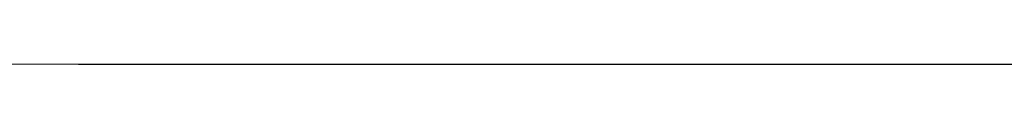
# Model space of a CAD drawing. Units: inches. Extents: x 459864 to 460310, y 324185 to 324787.
# Tile 97 of 112: x 460247.676 to 460248.739, y 324283.483 to 324283.483. Entities that reach past the tile are written whole.
import ezdxf

# ---------------------------------------------------------------- set-up
doc = ezdxf.new("R2010")
doc.units = ezdxf.units.IN
for name, color, linetype, lineweight in [('A-ANNO-DIMS', 2, 'Continuous', 18), ('L-HRDS', 9, 'Continuous', 18), ('L-SITE-PATT', 252, 'Continuous', 13)]:
    doc.layers.add(name, color=color, linetype=linetype, lineweight=lineweight)
doc.styles.get("Standard").update_dxf_attribs({"font": 'arial.ttf'})
doc.dimstyles.new('ISO-25', dxfattribs={"dimtxt": 6, "dimasz": 2.5, "dimexe": 1.25, "dimexo": 0.625, "dimtad": 1, "dimdec": 1, "dimlunit": 3, "dimtxsty": 'Standard', "dimcen": 2.5, "dimadec": 0, "dimazin": 0, "dimtfac": 1, "dimtdec": 1, "dimtmove": 0, "dimatfit": 3, "dimfxl": 1, "dimarcsym": 0})

# ---------------------------------------------------------------- blocks, each defined once
blk = doc.blocks.new('*D21')
at = {"layer": 'A-ANNO-DIMS', "color": 0, "lineweight": -2, "transparency": 16777216}
for p, q in [((460247.7399, 324715.4832), (460309.5804, 324715.4832)), ((460308.3304, 324712.9832), (460308.3304, 324285.9832)), ((460247.7399, 324283.4832), (460309.5804, 324283.4832))]:
    blk.add_line(p, q, dxfattribs=at)
at = {"layer": 'A-ANNO-DIMS', "color": 0, "transparency": 16777216}
for points in [[(460307.9137, 324712.9832), (460308.747, 324712.9832), (460308.3304, 324715.4832)], [(460307.9137, 324285.9832), (460308.747, 324285.9832), (460308.3304, 324283.4832)]]:
    blk.add_solid(points, dxfattribs=at)
at = {"layer": 'Defpoints', "color": 0, "transparency": 16777216}
for p in [(460247.1149, 324715.4832), (460247.1149, 324283.4832), (460308.3304, 324283.4832)]:
    blk.add_point(p, dxfattribs=at)
at = {"layer": 'A-ANNO-DIMS', "color": 0, "transparency": 16777216, "insert": (460304.6399, 324499.4832), "char_height": 6, "attachment_point": 5, "rotation": 90}
blk.add_mtext("36'", dxfattribs=at)

msp = doc.modelspace()

# ---------------------------------------------------------------- hatches: boundary and pattern name
at = {"layer": 'L-SITE-PATT'}
h = msp.add_hatch(dxfattribs=at)
h.set_pattern_fill('DOTS', color=256)
h.paths.add_polyline_path([(460269.8036, 324283.4832), (460247.1149, 324283.4832), (460121.9293, 324283.4832), (460121.9293, 324252.473), (460117.4293, 324252.473), (460110.1236, 324252.473), (460110.1236, 324243.2865), (460080.8295, 324243.2865), (460080.8295, 324252.473), (460061.1149, 324252.473), (460061.1149, 324251.8824), (460077.9089, 324251.8824), (460077.9089, 324199.4832), (460080.8295, 324199.4832), (460080.8295, 324207.5532), (460110.1236, 324207.5532), (460110.1236, 324199.4832), (460110.8133, 324199.4832), (460262.1149, 324199.4832), (460269.8036, 324199.4832)], flags=17)
edge = h.paths.add_edge_path(flags=0)
edge.add_ellipse((460222.5903, 324263.8132), major_axis=(-8.4853, 8.4853), ratio=1, start_angle=405, end_angle=495, ccw=False)
edge.add_line((460214.8209, 324254.6599), (460214.8316, 324254.6659))
edge.add_ellipse((460222.5903, 324263.8132), major_axis=(-8.4853, 8.4853), ratio=1, start_angle=405, end_angle=495, ccw=False)
edge.add_line((460210.7589, 324261.7806), (460210.7676, 324261.7868))
edge.add_ellipse((460222.5903, 324263.8132), major_axis=(-8.4853, 8.4853), ratio=1, start_angle=405, end_angle=495, ccw=False)
edge.add_ellipse((460222.5903, 324263.8132), major_axis=(-8.4853, 8.4853), ratio=1, start_angle=392.75402, end_angle=405, ccw=False)
edge.add_ellipse((460222.5903, 324263.8132), major_axis=(-8.4853, 8.4853), ratio=1, start_angle=380.93472, end_angle=392.75402, ccw=False)
edge.add_line((460211.3371, 324267.985), (460211.3404, 324267.985))
edge.add_ellipse((460222.5903, 324263.8132), major_axis=(-8.4853, 8.4853), ratio=1, start_angle=380.93472, end_angle=392.75402, ccw=False)
edge.add_ellipse((460222.5903, 324263.8132), major_axis=(-8.4853, 8.4853), ratio=1, start_angle=347.90152, end_angle=380.93472, ccw=False)
edge.add_ellipse((460222.5903, 324263.8132), major_axis=(-8.4853, 8.4853), ratio=1, start_angle=327.06192, end_angle=347.90152, ccw=False)
edge.add_ellipse((460222.5903, 324263.8132), major_axis=(-8.4853, 8.4853), ratio=1, start_angle=278.32464, end_angle=327.06192, ccw=False)
edge.add_line((460225.1583, 324275.536), (460225.1577, 324275.5346))
edge.add_ellipse((460222.5903, 324263.8132), major_axis=(-8.4853, 8.4853), ratio=1, start_angle=278.32464, end_angle=327.06192, ccw=False)
edge.add_ellipse((460222.5903, 324263.8132), major_axis=(-8.4853, 8.4853), ratio=1, start_angle=260.64357, end_angle=278.32464, ccw=False)
edge.add_ellipse((460222.5903, 324263.8132), major_axis=(-8.4853, 8.4853), ratio=1, start_angle=225, end_angle=260.64357, ccw=False)
edge.add_line((460234.5088, 324265.2428), (460234.5015, 324265.2394))
edge.add_ellipse((460222.5903, 324263.8132), major_axis=(-8.4853, 8.4853), ratio=1, start_angle=225, end_angle=260.64357, ccw=False)
edge.add_ellipse((460222.5903, 324263.8132), major_axis=(-8.4853, 8.4853), ratio=1, start_angle=495, end_angle=585, ccw=False)
edge.add_line((460234.4367, 324261.8612), (460234.4238, 324261.8578))
edge.add_ellipse((460222.5903, 324263.8132), major_axis=(-8.4853, 8.4853), ratio=1, start_angle=495, end_angle=585, ccw=False)
edge.add_line((460227.9501, 324253.0672), (460227.9464, 324253.0831))
edge.add_ellipse((460222.5903, 324263.8132), major_axis=(-8.4853, 8.4853), ratio=1, start_angle=495, end_angle=585, ccw=False)
edge.add_line((460226.223, 324252.3693), (460226.211, 324252.3796))
edge.add_ellipse((460222.5903, 324263.8132), major_axis=(-8.4853, 8.4853), ratio=1, start_angle=495, end_angle=585, ccw=False)
h.paths.add_polyline_path([(460219.6515, 324254.3467), (460218.4613, 324253.545), (460218.2754, 324254.7893), (460219.6424, 324256.5418), (460219.6246, 324260.8476), (460216.1101, 324257.333), (460214.35, 324256.9781), (460215.4164, 324259.3557), (460212.5239, 324258.4958), (460213.1373, 324259.9298), (460218.5072, 324263.8132), (460222.5903, 324263.8132), (460222.5903, 324267.8067), (460218.1755, 324272.2123), (460219.026, 324274.639), (460222.5903, 324272.8111), (460222.5903, 324275.4233), (460223.0571, 324274.8249), (460222.6752, 324273.4922), (460225.9117, 324267.1346), (460219.6246, 324260.8476)], flags=0)
edge = h.paths.add_edge_path(flags=0)
edge.add_ellipse((460194.5758, 324264.0465), major_axis=(-8.4853, 8.4853), ratio=1, start_angle=495, end_angle=585, ccw=False)
edge.add_line((460199.9356, 324253.3005), (460199.9319, 324253.3164))
edge.add_ellipse((460194.5758, 324264.0465), major_axis=(-8.4853, 8.4853), ratio=1, start_angle=495, end_angle=585, ccw=False)
edge.add_line((460198.2084, 324252.6025), (460198.1965, 324252.6128))
edge.add_ellipse((460194.5758, 324264.0465), major_axis=(-8.4853, 8.4853), ratio=1, start_angle=495, end_angle=585, ccw=False)
edge.add_ellipse((460194.5758, 324264.0465), major_axis=(-8.4853, 8.4853), ratio=1, start_angle=405, end_angle=495, ccw=False)
edge.add_line((460186.8063, 324254.8932), (460186.8171, 324254.8992))
edge.add_ellipse((460194.5758, 324264.0465), major_axis=(-8.4853, 8.4853), ratio=1, start_angle=405, end_angle=495, ccw=False)
edge.add_line((460182.7444, 324262.0138), (460182.753, 324262.0201))
edge.add_ellipse((460194.5758, 324264.0465), major_axis=(-8.4853, 8.4853), ratio=1, start_angle=405, end_angle=495, ccw=False)
edge.add_ellipse((460194.5758, 324264.0465), major_axis=(-8.4853, 8.4853), ratio=1, start_angle=392.75402, end_angle=405, ccw=False)
edge.add_ellipse((460194.5758, 324264.0465), major_axis=(-8.4853, 8.4853), ratio=1, start_angle=380.93472, end_angle=392.75402, ccw=False)
edge.add_line((460183.3225, 324268.2183), (460183.3259, 324268.2183))
edge.add_ellipse((460194.5758, 324264.0465), major_axis=(-8.4853, 8.4853), ratio=1, start_angle=380.93472, end_angle=392.75402, ccw=False)
edge.add_ellipse((460194.5758, 324264.0465), major_axis=(-8.4853, 8.4853), ratio=1, start_angle=347.90152, end_angle=380.93472, ccw=False)
edge.add_ellipse((460194.5758, 324264.0465), major_axis=(-8.4853, 8.4853), ratio=1, start_angle=327.06192, end_angle=347.90152, ccw=False)
edge.add_ellipse((460194.5758, 324264.0465), major_axis=(-8.4853, 8.4853), ratio=1, start_angle=278.32464, end_angle=327.06192, ccw=False)
edge.add_line((460197.1437, 324275.7693), (460197.1432, 324275.7679))
edge.add_ellipse((460194.5758, 324264.0465), major_axis=(-8.4853, 8.4853), ratio=1, start_angle=278.32464, end_angle=327.06192, ccw=False)
edge.add_ellipse((460194.5758, 324264.0465), major_axis=(-8.4853, 8.4853), ratio=1, start_angle=260.64357, end_angle=278.32464, ccw=False)
edge.add_ellipse((460194.5758, 324264.0465), major_axis=(-8.4853, 8.4853), ratio=1, start_angle=225, end_angle=260.64357, ccw=False)
edge.add_line((460206.4943, 324265.4761), (460206.4869, 324265.4727))
edge.add_ellipse((460194.5758, 324264.0465), major_axis=(-8.4853, 8.4853), ratio=1, start_angle=225, end_angle=260.64357, ccw=False)
edge.add_ellipse((460194.5758, 324264.0465), major_axis=(-8.4853, 8.4853), ratio=1, start_angle=495, end_angle=585, ccw=False)
edge.add_line((460206.4221, 324262.0945), (460206.4092, 324262.0911))
h.paths.add_polyline_path([(460191.6101, 324261.0808), (460191.6369, 324254.5799), (460190.4468, 324253.7783), (460190.2609, 324255.0226), (460191.6279, 324256.775), (460191.6101, 324261.0808), (460188.0956, 324257.5663), (460186.3354, 324257.2113), (460187.4018, 324259.5889), (460184.5094, 324258.7291), (460185.1228, 324260.1631), (460190.4927, 324264.0465), (460194.5758, 324264.0465), (460194.5758, 324268.04), (460190.161, 324272.4456), (460191.0114, 324274.8722), (460194.5758, 324273.0444), (460194.5758, 324275.6566), (460195.0426, 324275.0582), (460194.6607, 324273.7255), (460197.8971, 324267.3679)], flags=0)
edge = h.paths.add_edge_path(flags=0)
edge.add_ellipse((460252.912, 324263.5776), major_axis=(-8.4853, 8.4853), ratio=1, start_angle=405, end_angle=495, ccw=False)
edge.add_line((460241.0806, 324261.5449), (460241.0892, 324261.5512))
edge.add_ellipse((460252.912, 324263.5776), major_axis=(-8.4853, 8.4853), ratio=1, start_angle=405, end_angle=495, ccw=False)
edge.add_ellipse((460252.912, 324263.5776), major_axis=(-8.4853, 8.4853), ratio=1, start_angle=392.75402, end_angle=405, ccw=False)
edge.add_ellipse((460252.912, 324263.5776), major_axis=(-8.4853, 8.4853), ratio=1, start_angle=380.93472, end_angle=392.75402, ccw=False)
edge.add_line((460241.6587, 324267.7494), (460241.6621, 324267.7494))
edge.add_ellipse((460252.912, 324263.5776), major_axis=(-8.4853, 8.4853), ratio=1, start_angle=380.93472, end_angle=392.75402, ccw=False)
edge.add_ellipse((460252.912, 324263.5776), major_axis=(-8.4853, 8.4853), ratio=1, start_angle=347.90152, end_angle=380.93472, ccw=False)
edge.add_ellipse((460252.912, 324263.5776), major_axis=(-8.4853, 8.4853), ratio=1, start_angle=327.06192, end_angle=347.90152, ccw=False)
edge.add_ellipse((460252.912, 324263.5776), major_axis=(-8.4853, 8.4853), ratio=1, start_angle=278.32464, end_angle=327.06192, ccw=False)
edge.add_line((460255.4799, 324275.3004), (460255.4794, 324275.299))
edge.add_ellipse((460252.912, 324263.5776), major_axis=(-8.4853, 8.4853), ratio=1, start_angle=278.32464, end_angle=327.06192, ccw=False)
edge.add_ellipse((460252.912, 324263.5776), major_axis=(-8.4853, 8.4853), ratio=1, start_angle=260.64357, end_angle=278.32464, ccw=False)
edge.add_ellipse((460252.912, 324263.5776), major_axis=(-8.4853, 8.4853), ratio=1, start_angle=225, end_angle=260.64357, ccw=False)
edge.add_line((460264.8305, 324265.0072), (460264.8231, 324265.0038))
edge.add_ellipse((460252.912, 324263.5776), major_axis=(-8.4853, 8.4853), ratio=1, start_angle=225, end_angle=260.64357, ccw=False)
edge.add_ellipse((460252.912, 324263.5776), major_axis=(-8.4853, 8.4853), ratio=1, start_angle=495, end_angle=585, ccw=False)
edge.add_line((460264.7583, 324261.6256), (460264.7454, 324261.6222))
edge.add_ellipse((460252.912, 324263.5776), major_axis=(-8.4853, 8.4853), ratio=1, start_angle=495, end_angle=585, ccw=False)
edge.add_line((460258.2718, 324252.8316), (460258.2681, 324252.8475))
edge.add_ellipse((460252.912, 324263.5776), major_axis=(-8.4853, 8.4853), ratio=1, start_angle=495, end_angle=585, ccw=False)
edge.add_line((460256.5446, 324252.1337), (460256.5327, 324252.1439))
edge.add_ellipse((460252.912, 324263.5776), major_axis=(-8.4853, 8.4853), ratio=1, start_angle=495, end_angle=585, ccw=False)
edge.add_ellipse((460252.912, 324263.5776), major_axis=(-8.4853, 8.4853), ratio=1, start_angle=405, end_angle=495, ccw=False)
edge.add_line((460245.1425, 324254.4243), (460245.1533, 324254.4303))
h.paths.add_polyline_path([(460244.6716, 324256.7425), (460245.738, 324259.1201), (460242.8456, 324258.2602), (460243.459, 324259.6942), (460248.8289, 324263.5776), (460252.912, 324263.5776), (460252.912, 324267.5711), (460248.4972, 324271.9767), (460249.3476, 324274.4034), (460252.912, 324272.5755), (460252.912, 324275.1877), (460253.3788, 324274.5893), (460252.9969, 324273.2566), (460256.2333, 324266.899), (460249.9463, 324260.612), (460249.9731, 324254.111), (460248.783, 324253.3094), (460248.5971, 324254.5537), (460249.9641, 324256.3062), (460249.9463, 324260.612), (460246.4318, 324257.0974)], flags=0)
edge = h.paths.add_edge_path(flags=0)
edge.add_ellipse((460167.4387, 324262.8328), major_axis=(-8.4853, 8.4853), ratio=1, start_angle=495, end_angle=585, ccw=False)
edge.add_line((460172.7985, 324252.0868), (460172.7948, 324252.1027))
edge.add_ellipse((460167.4387, 324262.8328), major_axis=(-8.4853, 8.4853), ratio=1, start_angle=495, end_angle=585, ccw=False)
edge.add_line((460171.0714, 324251.3888), (460171.0594, 324251.3991))
edge.add_ellipse((460167.4387, 324262.8328), major_axis=(-8.4853, 8.4853), ratio=1, start_angle=495, end_angle=585, ccw=False)
edge.add_ellipse((460167.4387, 324262.8328), major_axis=(-8.4853, 8.4853), ratio=1, start_angle=405, end_angle=495, ccw=False)
edge.add_line((460159.6693, 324253.6795), (460159.68, 324253.6855))
edge.add_ellipse((460167.4387, 324262.8328), major_axis=(-8.4853, 8.4853), ratio=1, start_angle=405, end_angle=495, ccw=False)
edge.add_line((460155.6073, 324260.8001), (460155.616, 324260.8064))
edge.add_ellipse((460167.4387, 324262.8328), major_axis=(-8.4853, 8.4853), ratio=1, start_angle=405, end_angle=495, ccw=False)
edge.add_ellipse((460167.4387, 324262.8328), major_axis=(-8.4853, 8.4853), ratio=1, start_angle=392.75402, end_angle=405, ccw=False)
edge.add_ellipse((460167.4387, 324262.8328), major_axis=(-8.4853, 8.4853), ratio=1, start_angle=380.93472, end_angle=392.75402, ccw=False)
edge.add_line((460156.1855, 324267.0046), (460156.1888, 324267.0046))
edge.add_ellipse((460167.4387, 324262.8328), major_axis=(-8.4853, 8.4853), ratio=1, start_angle=380.93472, end_angle=392.75402, ccw=False)
edge.add_ellipse((460167.4387, 324262.8328), major_axis=(-8.4853, 8.4853), ratio=1, start_angle=347.90152, end_angle=380.93472, ccw=False)
edge.add_ellipse((460167.4387, 324262.8328), major_axis=(-8.4853, 8.4853), ratio=1, start_angle=327.06192, end_angle=347.90152, ccw=False)
edge.add_ellipse((460167.4387, 324262.8328), major_axis=(-8.4853, 8.4853), ratio=1, start_angle=278.32464, end_angle=327.06192, ccw=False)
edge.add_line((460170.0067, 324274.5556), (460170.0061, 324274.5542))
edge.add_ellipse((460167.4387, 324262.8328), major_axis=(-8.4853, 8.4853), ratio=1, start_angle=278.32464, end_angle=327.06192, ccw=False)
edge.add_ellipse((460167.4387, 324262.8328), major_axis=(-8.4853, 8.4853), ratio=1, start_angle=260.64357, end_angle=278.32464, ccw=False)
edge.add_ellipse((460167.4387, 324262.8328), major_axis=(-8.4853, 8.4853), ratio=1, start_angle=225, end_angle=260.64357, ccw=False)
edge.add_line((460179.3572, 324264.2624), (460179.3499, 324264.259))
edge.add_ellipse((460167.4387, 324262.8328), major_axis=(-8.4853, 8.4853), ratio=1, start_angle=225, end_angle=260.64357, ccw=False)
edge.add_ellipse((460167.4387, 324262.8328), major_axis=(-8.4853, 8.4853), ratio=1, start_angle=495, end_angle=585, ccw=False)
edge.add_line((460179.2851, 324260.8808), (460179.2722, 324260.8774))
h.paths.add_polyline_path([(460164.473, 324259.8671), (460164.4998, 324253.3662), (460163.3097, 324252.5645), (460163.1238, 324253.8089), (460164.4908, 324255.5613), (460164.473, 324259.8671), (460160.9585, 324256.3526), (460159.1984, 324255.9976), (460160.2648, 324258.3752), (460157.3723, 324257.5154), (460157.9857, 324258.9494), (460163.3556, 324262.8328), (460167.4387, 324262.8328), (460167.4387, 324266.8263), (460163.0239, 324271.2319), (460163.8744, 324273.6585), (460167.4387, 324271.8307), (460167.4387, 324274.4429), (460167.9055, 324273.8445), (460167.5236, 324272.5118), (460170.7601, 324266.1542)], flags=0)
edge = h.paths.add_edge_path(flags=0)
edge.add_ellipse((460140.7581, 324262.3696), major_axis=(-8.4853, 8.4853), ratio=1, start_angle=495, end_angle=585, ccw=False)
edge.add_line((460146.1179, 324251.6235), (460146.1142, 324251.6395))
edge.add_ellipse((460140.7581, 324262.3696), major_axis=(-8.4853, 8.4853), ratio=1, start_angle=495, end_angle=585, ccw=False)
edge.add_line((460144.3908, 324250.9256), (460144.3788, 324250.9359))
edge.add_ellipse((460140.7581, 324262.3696), major_axis=(-8.4853, 8.4853), ratio=1, start_angle=495, end_angle=585, ccw=False)
edge.add_ellipse((460140.7581, 324262.3696), major_axis=(-8.4853, 8.4853), ratio=1, start_angle=405, end_angle=495, ccw=False)
edge.add_line((460132.9887, 324253.2162), (460132.9994, 324253.2223))
edge.add_ellipse((460140.7581, 324262.3696), major_axis=(-8.4853, 8.4853), ratio=1, start_angle=405, end_angle=495, ccw=False)
edge.add_line((460128.9267, 324260.3369), (460128.9354, 324260.3432))
edge.add_ellipse((460140.7581, 324262.3696), major_axis=(-8.4853, 8.4853), ratio=1, start_angle=405, end_angle=495, ccw=False)
edge.add_ellipse((460140.7581, 324262.3696), major_axis=(-8.4853, 8.4853), ratio=1, start_angle=392.75402, end_angle=405, ccw=False)
edge.add_ellipse((460140.7581, 324262.3696), major_axis=(-8.4853, 8.4853), ratio=1, start_angle=380.93472, end_angle=392.75402, ccw=False)
edge.add_line((460129.5049, 324266.5414), (460129.5082, 324266.5414))
edge.add_ellipse((460140.7581, 324262.3696), major_axis=(-8.4853, 8.4853), ratio=1, start_angle=380.93472, end_angle=392.75402, ccw=False)
edge.add_ellipse((460140.7581, 324262.3696), major_axis=(-8.4853, 8.4853), ratio=1, start_angle=347.90152, end_angle=380.93472, ccw=False)
edge.add_ellipse((460140.7581, 324262.3696), major_axis=(-8.4853, 8.4853), ratio=1, start_angle=327.06192, end_angle=347.90152, ccw=False)
edge.add_ellipse((460140.7581, 324262.3696), major_axis=(-8.4853, 8.4853), ratio=1, start_angle=278.32464, end_angle=327.06192, ccw=False)
edge.add_line((460143.3261, 324274.0923), (460143.3255, 324274.091))
edge.add_ellipse((460140.7581, 324262.3696), major_axis=(-8.4853, 8.4853), ratio=1, start_angle=278.32464, end_angle=327.06192, ccw=False)
edge.add_ellipse((460140.7581, 324262.3696), major_axis=(-8.4853, 8.4853), ratio=1, start_angle=260.64357, end_angle=278.32464, ccw=False)
edge.add_ellipse((460140.7581, 324262.3696), major_axis=(-8.4853, 8.4853), ratio=1, start_angle=225, end_angle=260.64357, ccw=False)
edge.add_line((460152.6766, 324263.7992), (460152.6692, 324263.7958))
edge.add_ellipse((460140.7581, 324262.3696), major_axis=(-8.4853, 8.4853), ratio=1, start_angle=225, end_angle=260.64357, ccw=False)
edge.add_ellipse((460140.7581, 324262.3696), major_axis=(-8.4853, 8.4853), ratio=1, start_angle=495, end_angle=585, ccw=False)
edge.add_line((460152.6045, 324260.4176), (460152.5916, 324260.4142))
h.paths.add_polyline_path([(460137.7924, 324259.4039), (460137.8192, 324252.903), (460136.6291, 324252.1013), (460136.4432, 324253.3457), (460137.8102, 324255.0981), (460137.7924, 324259.4039), (460134.2779, 324255.8894), (460132.5178, 324255.5344), (460133.5842, 324257.912), (460130.6917, 324257.0522), (460131.3051, 324258.4862), (460136.675, 324262.3696), (460140.7581, 324262.3696), (460140.7581, 324266.3631), (460136.3433, 324270.7687), (460137.1938, 324273.1953), (460140.7581, 324271.3675), (460140.7581, 324273.9797), (460141.2249, 324273.3813), (460140.843, 324272.0486), (460144.0795, 324265.691)], flags=0)
h.paths.add_polyline_path([(460110.1236, 324227.4139), (460080.8295, 324227.4139), (460080.8295, 324235.4839), (460110.1236, 324235.4839)], flags=16)
h.paths.add_polyline_path([(460110.1236, 324220.7966), (460110.1236, 324212.7267), (460080.8295, 324212.7267), (460080.8295, 324220.7966)], flags=16)
h.paths.add_polyline_path([(460269.8036, 324283.4832), (460247.1149, 324283.4832), (460121.9293, 324283.4832), (460121.9293, 324252.473), (460117.4293, 324252.473), (460110.1236, 324252.473), (460110.1236, 324243.2865), (460080.8295, 324243.2865), (460080.8295, 324252.473), (460061.1149, 324252.473), (460061.1149, 324251.8824), (460077.9089, 324251.8824), (460077.9089, 324199.4832), (460080.8295, 324199.4832), (460080.8295, 324207.5532), (460110.1236, 324207.5532), (460110.1236, 324199.4832), (460262.1149, 324199.4832), (460269.8036, 324199.4832)], flags=17)
h.paths.add_polyline_path([(460219.6515, 324254.3467), (460218.4613, 324253.545), (460218.2754, 324254.7893), (460219.6424, 324256.5418), (460219.6246, 324260.8476), (460216.1101, 324257.333), (460214.35, 324256.9781), (460215.4164, 324259.3557), (460212.5239, 324258.4958), (460213.1373, 324259.9298), (460218.5072, 324263.8132), (460222.5903, 324263.8132), (460220.1805, 324266.223), (460215.461, 324265.3076), (460211.8345, 324266.1366), (460216.2466, 324267.985), (460218.4185, 324267.985), (460222.5903, 324263.8132), (460222.5903, 324267.8067), (460218.1755, 324272.2123), (460219.026, 324274.639), (460222.5903, 324272.8111), (460222.5903, 324275.4233), (460223.0571, 324274.8249), (460222.6752, 324273.4922), (460225.9117, 324267.1346), (460222.5903, 324263.8132), (460231.3829, 324263.8132), (460228.4847, 324262.4878), (460224.4252, 324261.9783), (460228.6799, 324257.7236), (460228.9658, 324254.791), (460227.1418, 324256.5366), (460227.5421, 324254.8186), (460227.3333, 324253.6145), (460222.5903, 324259.9846), (460222.5903, 324255.4967), (460221.3774, 324256.5408), (460220.5758, 324261.7987), (460219.6246, 324260.8476)], flags=0)
h.paths.add_polyline_path([(460199.1272, 324256.7699), (460199.5275, 324255.0518), (460199.3188, 324253.8477), (460194.5758, 324260.2179), (460194.5758, 324255.7299), (460193.3629, 324256.7741), (460192.5613, 324262.032), (460191.6101, 324261.0808), (460191.6369, 324254.5799), (460190.4468, 324253.7783), (460190.2609, 324255.0226), (460191.6279, 324256.775), (460191.6101, 324261.0808), (460188.0956, 324257.5663), (460186.3354, 324257.2113), (460187.4018, 324259.5889), (460184.5094, 324258.7291), (460185.1228, 324260.1631), (460190.4927, 324264.0465), (460194.5758, 324264.0465), (460192.1659, 324266.4563), (460187.4464, 324265.5409), (460183.82, 324266.3698), (460188.2321, 324268.2183), (460190.404, 324268.2183), (460194.5758, 324264.0465), (460194.5758, 324268.04), (460190.161, 324272.4456), (460191.0114, 324274.8722), (460194.5758, 324273.0444), (460194.5758, 324275.6566), (460195.0426, 324275.0582), (460194.6607, 324273.7255), (460197.8971, 324267.3679), (460194.5758, 324264.0465), (460203.3683, 324264.0465), (460200.4702, 324262.7211), (460196.4107, 324262.2116), (460200.6654, 324257.9569), (460200.9513, 324255.0243)], flags=0)
h.paths.add_polyline_path([(460244.6716, 324256.7425), (460245.738, 324259.1201), (460242.8456, 324258.2602), (460243.459, 324259.6942), (460248.8289, 324263.5776), (460252.912, 324263.5776), (460250.5022, 324265.9874), (460245.7826, 324265.072), (460242.1562, 324265.9009), (460246.5683, 324267.7494), (460248.7402, 324267.7494), (460252.912, 324263.5776), (460252.912, 324267.5711), (460248.4972, 324271.9767), (460249.3476, 324274.4034), (460252.912, 324272.5755), (460252.912, 324275.1877), (460253.3788, 324274.5893), (460252.9969, 324273.2566), (460256.2333, 324266.899), (460252.912, 324263.5776), (460261.7045, 324263.5776), (460258.8064, 324262.2522), (460254.7469, 324261.7427), (460259.0016, 324257.488), (460259.2875, 324254.5554), (460257.4634, 324256.301), (460257.8637, 324254.583), (460257.655, 324253.3789), (460252.912, 324259.749), (460252.912, 324255.2611), (460251.6991, 324256.3052), (460250.8975, 324261.5631), (460249.9463, 324260.612), (460249.9731, 324254.111), (460248.783, 324253.3094), (460248.5971, 324254.5537), (460249.9641, 324256.3062), (460249.9463, 324260.612), (460246.4318, 324257.0974)], flags=0)
h.paths.add_polyline_path([(460173.5283, 324256.7432), (460173.8142, 324253.8106), (460171.9902, 324255.5562), (460172.3905, 324253.8381), (460172.1817, 324252.634), (460167.4387, 324259.0042), (460167.4387, 324254.5162), (460166.2258, 324255.5604), (460165.4242, 324260.8183), (460164.473, 324259.8671), (460164.4998, 324253.3662), (460163.3097, 324252.5645), (460163.1238, 324253.8089), (460164.4908, 324255.5613), (460164.473, 324259.8671), (460160.9585, 324256.3526), (460159.1984, 324255.9976), (460160.2648, 324258.3752), (460157.3723, 324257.5154), (460157.9857, 324258.9494), (460163.3556, 324262.8328), (460167.4387, 324262.8328), (460165.0289, 324265.2426), (460160.3094, 324264.3272), (460156.6829, 324265.1561), (460161.095, 324267.0046), (460163.2669, 324267.0046), (460167.4387, 324262.8328), (460167.4387, 324266.8263), (460163.0239, 324271.2319), (460163.8744, 324273.6585), (460167.4387, 324271.8307), (460167.4387, 324274.4429), (460167.9055, 324273.8445), (460167.5236, 324272.5118), (460170.7601, 324266.1542), (460167.4387, 324262.8328), (460176.2313, 324262.8328), (460173.3331, 324261.5074), (460169.2736, 324260.9979)], flags=0)
h.paths.add_polyline_path([(460146.8477, 324256.28), (460147.1336, 324253.3474), (460145.3096, 324255.093), (460145.7099, 324253.3749), (460145.5011, 324252.1708), (460140.7581, 324258.541), (460140.7581, 324254.053), (460139.5452, 324255.0972), (460138.7436, 324260.3551), (460137.7924, 324259.4039), (460137.8192, 324252.903), (460136.6291, 324252.1013), (460136.4432, 324253.3457), (460137.8102, 324255.0981), (460137.7924, 324259.4039), (460134.2779, 324255.8894), (460132.5178, 324255.5344), (460133.5842, 324257.912), (460130.6917, 324257.0522), (460131.3051, 324258.4862), (460136.675, 324262.3696), (460140.7581, 324262.3696), (460138.3483, 324264.7794), (460133.6288, 324263.864), (460130.0023, 324264.6929), (460134.4144, 324266.5414), (460136.5863, 324266.5414), (460140.7581, 324262.3696), (460140.7581, 324266.3631), (460136.3433, 324270.7687), (460137.1938, 324273.1953), (460140.7581, 324271.3675), (460140.7581, 324273.9797), (460141.2249, 324273.3813), (460140.843, 324272.0486), (460144.0795, 324265.691), (460140.7581, 324262.3696), (460149.5507, 324262.3696), (460146.6525, 324261.0442), (460142.593, 324260.5347)], flags=0)
edge = h.paths.add_edge_path()
edge.add_line((460269.8036, 324272.5491), (460260.8815, 324272.5491))
edge.add_ellipse((460252.912, 324263.5776), major_axis=(-8.4853, 8.4853), ratio=1, start_angle=260.64357, end_angle=273.38462, ccw=False)
edge.add_line((460262.2826, 324271.0921), (460262.2606, 324271.0911))
edge.add_ellipse((460252.912, 324263.5776), major_axis=(-8.4853, 8.4853), ratio=1, start_angle=260.64357, end_angle=273.38462, ccw=False)
edge.add_ellipse((460252.912, 324263.5776), major_axis=(-8.4853, 8.4853), ratio=1, start_angle=225, end_angle=260.64357, ccw=False)
edge.add_line((460263.6086, 324269.0633), (460263.5717, 324269.0583))
edge.add_ellipse((460252.912, 324263.5776), major_axis=(-8.4853, 8.4853), ratio=1, start_angle=225, end_angle=260.64357, ccw=False)
edge.add_line((460264.6155, 324266.3055), (460264.5854, 324266.3052))
edge.add_ellipse((460252.912, 324263.5776), major_axis=(-8.4853, 8.4853), ratio=1, start_angle=225, end_angle=260.64357, ccw=False)
edge.add_line((460264.8305, 324265.0072), (460264.8231, 324265.0038))
edge.add_ellipse((460252.912, 324263.5776), major_axis=(-8.4853, 8.4853), ratio=1, start_angle=225, end_angle=260.64357, ccw=False)
edge.add_ellipse((460252.912, 324263.5776), major_axis=(-8.4853, 8.4853), ratio=1, start_angle=495, end_angle=585, ccw=False)
edge.add_line((460264.7583, 324261.6256), (460264.7454, 324261.6222))
edge.add_ellipse((460252.912, 324263.5776), major_axis=(-8.4853, 8.4853), ratio=1, start_angle=495, end_angle=585, ccw=False)
edge.add_line((460263.4422, 324257.739), (460263.3893, 324257.7792))
edge.add_ellipse((460252.912, 324263.5776), major_axis=(-8.4853, 8.4853), ratio=1, start_angle=495, end_angle=585, ccw=False)
edge.add_line((460258.1281, 324252.7435), (460258.1019, 324252.7787))
edge.add_ellipse((460252.912, 324263.5776), major_axis=(-8.4853, 8.4853), ratio=1, start_angle=495, end_angle=585, ccw=False)
edge.add_line((460256.5446, 324252.1337), (460256.5327, 324252.1439))
edge.add_ellipse((460252.912, 324263.5776), major_axis=(-8.4853, 8.4853), ratio=1, start_angle=495, end_angle=585, ccw=False)
edge.add_ellipse((460252.912, 324263.5776), major_axis=(-8.4853, 8.4853), ratio=1, start_angle=405, end_angle=495, ccw=False)
edge.add_line((460250.594, 324251.7804), (460250.6047, 324251.8198))
edge.add_ellipse((460252.912, 324263.5776), major_axis=(-8.4853, 8.4853), ratio=1, start_angle=405, end_angle=495, ccw=False)
edge.add_line((460245.1425, 324254.4243), (460245.1533, 324254.4303))
edge.add_ellipse((460252.912, 324263.5776), major_axis=(-8.4853, 8.4853), ratio=1, start_angle=405, end_angle=495, ccw=False)
edge.add_line((460243.5246, 324256.059), (460243.5603, 324256.0914))
edge.add_ellipse((460252.912, 324263.5776), major_axis=(-8.4853, 8.4853), ratio=1, start_angle=405, end_angle=495, ccw=False)
edge.add_line((460241.4401, 324259.8927), (460241.5224, 324259.8959))
edge.add_ellipse((460252.912, 324263.5776), major_axis=(-8.4853, 8.4853), ratio=1, start_angle=405, end_angle=495, ccw=False)
edge.add_line((460241.0806, 324261.5449), (460241.0892, 324261.5512))
edge.add_ellipse((460252.912, 324263.5776), major_axis=(-8.4853, 8.4853), ratio=1, start_angle=405, end_angle=495, ccw=False)
edge.add_ellipse((460252.912, 324263.5776), major_axis=(-8.4853, 8.4853), ratio=1, start_angle=392.75402, end_angle=405, ccw=False)
edge.add_line((460241.0503, 324265.4376), (460241.0626, 324265.4428))
edge.add_ellipse((460252.912, 324263.5776), major_axis=(-8.4853, 8.4853), ratio=1, start_angle=392.75402, end_angle=405, ccw=False)
edge.add_ellipse((460252.912, 324263.5776), major_axis=(-8.4853, 8.4853), ratio=1, start_angle=380.93472, end_angle=392.75402, ccw=False)
edge.add_line((460241.4519, 324267.1764), (460241.469, 324267.171))
edge.add_ellipse((460252.912, 324263.5776), major_axis=(-8.4853, 8.4853), ratio=1, start_angle=380.93472, end_angle=392.75402, ccw=False)
edge.add_line((460241.6587, 324267.7494), (460241.6621, 324267.7494))
edge.add_ellipse((460252.912, 324263.5776), major_axis=(-8.4853, 8.4853), ratio=1, start_angle=380.93472, end_angle=392.75402, ccw=False)
edge.add_ellipse((460252.912, 324263.5776), major_axis=(-8.4853, 8.4853), ratio=1, start_angle=356.61538, end_angle=380.93472, ccw=False)
edge.add_line((460244.8803, 324272.4877), (460244.7127, 324272.5491))
edge.add_line((460244.7127, 324272.5491), (460230.8174, 324272.5491))
edge.add_ellipse((460222.5903, 324263.8132), major_axis=(-8.4853, 8.4853), ratio=1, start_angle=260.64357, end_angle=271.71777, ccw=False)
edge.add_ellipse((460222.5903, 324263.8132), major_axis=(-8.4853, 8.4853), ratio=1, start_angle=225, end_angle=260.64357, ccw=False)
edge.add_line((460233.2869, 324269.2989), (460233.25, 324269.2939))
edge.add_ellipse((460222.5903, 324263.8132), major_axis=(-8.4853, 8.4853), ratio=1, start_angle=225, end_angle=260.64357, ccw=False)
edge.add_line((460234.2938, 324266.5412), (460234.2637, 324266.5408))
edge.add_ellipse((460222.5903, 324263.8132), major_axis=(-8.4853, 8.4853), ratio=1, start_angle=225, end_angle=260.64357, ccw=False)
edge.add_line((460234.5088, 324265.2428), (460234.5015, 324265.2394))
edge.add_ellipse((460222.5903, 324263.8132), major_axis=(-8.4853, 8.4853), ratio=1, start_angle=225, end_angle=260.64357, ccw=False)
edge.add_ellipse((460222.5903, 324263.8132), major_axis=(-8.4853, 8.4853), ratio=1, start_angle=495, end_angle=585, ccw=False)
edge.add_line((460234.4367, 324261.8612), (460234.4238, 324261.8578))
edge.add_ellipse((460222.5903, 324263.8132), major_axis=(-8.4853, 8.4853), ratio=1, start_angle=495, end_angle=585, ccw=False)
edge.add_line((460233.1205, 324257.9746), (460233.0676, 324258.0149))
edge.add_ellipse((460222.5903, 324263.8132), major_axis=(-8.4853, 8.4853), ratio=1, start_angle=495, end_angle=585, ccw=False)
edge.add_line((460227.8064, 324252.9791), (460227.7802, 324253.0143))
edge.add_ellipse((460222.5903, 324263.8132), major_axis=(-8.4853, 8.4853), ratio=1, start_angle=495, end_angle=585, ccw=False)
edge.add_line((460226.223, 324252.3693), (460226.211, 324252.3796))
edge.add_ellipse((460222.5903, 324263.8132), major_axis=(-8.4853, 8.4853), ratio=1, start_angle=495, end_angle=585, ccw=False)
edge.add_ellipse((460222.5903, 324263.8132), major_axis=(-8.4853, 8.4853), ratio=1, start_angle=405, end_angle=495, ccw=False)
edge.add_line((460220.2723, 324252.016), (460220.283, 324252.0554))
edge.add_ellipse((460222.5903, 324263.8132), major_axis=(-8.4853, 8.4853), ratio=1, start_angle=405, end_angle=495, ccw=False)
edge.add_line((460214.8209, 324254.6599), (460214.8316, 324254.6659))
edge.add_ellipse((460222.5903, 324263.8132), major_axis=(-8.4853, 8.4853), ratio=1, start_angle=405, end_angle=495, ccw=False)
edge.add_line((460213.2029, 324256.2946), (460213.2387, 324256.327))
edge.add_ellipse((460222.5903, 324263.8132), major_axis=(-8.4853, 8.4853), ratio=1, start_angle=405, end_angle=495, ccw=False)
edge.add_line((460211.1184, 324260.1283), (460211.2008, 324260.1315))
edge.add_ellipse((460222.5903, 324263.8132), major_axis=(-8.4853, 8.4853), ratio=1, start_angle=405, end_angle=495, ccw=False)
edge.add_line((460210.7589, 324261.7806), (460210.7676, 324261.7868))
edge.add_ellipse((460222.5903, 324263.8132), major_axis=(-8.4853, 8.4853), ratio=1, start_angle=405, end_angle=495, ccw=False)
edge.add_ellipse((460222.5903, 324263.8132), major_axis=(-8.4853, 8.4853), ratio=1, start_angle=392.75402, end_angle=405, ccw=False)
edge.add_line((460210.7286, 324265.6732), (460210.7409, 324265.6784))
edge.add_ellipse((460222.5903, 324263.8132), major_axis=(-8.4853, 8.4853), ratio=1, start_angle=392.75402, end_angle=405, ccw=False)
edge.add_ellipse((460222.5903, 324263.8132), major_axis=(-8.4853, 8.4853), ratio=1, start_angle=380.93472, end_angle=392.75402, ccw=False)
edge.add_line((460211.1302, 324267.412), (460211.1474, 324267.4066))
edge.add_ellipse((460222.5903, 324263.8132), major_axis=(-8.4853, 8.4853), ratio=1, start_angle=380.93472, end_angle=392.75402, ccw=False)
edge.add_line((460211.3371, 324267.985), (460211.3404, 324267.985))
edge.add_ellipse((460222.5903, 324263.8132), major_axis=(-8.4853, 8.4853), ratio=1, start_angle=380.93472, end_angle=392.75402, ccw=False)
edge.add_ellipse((460222.5903, 324263.8132), major_axis=(-8.4853, 8.4853), ratio=1, start_angle=358.28223, end_angle=380.93472, ccw=False)
edge.add_line((460213.7045, 324271.9018), (460213.709, 324271.869))
edge.add_ellipse((460222.5903, 324263.8132), major_axis=(-8.4853, 8.4853), ratio=1, start_angle=358.28223, end_angle=380.93472, ccw=False)
edge.add_line((460214.3632, 324272.5491), (460203.0783, 324272.5491))
edge.add_line((460203.0783, 324272.5491), (460203.0603, 324272.5311))
edge.add_ellipse((460194.5758, 324264.0465), major_axis=(-8.4853, 8.4853), ratio=1, start_angle=260.64357, end_angle=270.11679, ccw=False)
edge.add_line((460203.9566, 324271.5615), (460203.9209, 324271.5598))
edge.add_ellipse((460194.5758, 324264.0465), major_axis=(-8.4853, 8.4853), ratio=1, start_angle=260.64357, end_angle=270.11679, ccw=False)
edge.add_ellipse((460194.5758, 324264.0465), major_axis=(-8.4853, 8.4853), ratio=1, start_angle=225, end_angle=260.64357, ccw=False)
edge.add_line((460205.2724, 324269.5322), (460205.2354, 324269.5272))
edge.add_ellipse((460194.5758, 324264.0465), major_axis=(-8.4853, 8.4853), ratio=1, start_angle=225, end_angle=260.64357, ccw=False)
edge.add_line((460206.2793, 324266.7744), (460206.2492, 324266.7741))
edge.add_ellipse((460194.5758, 324264.0465), major_axis=(-8.4853, 8.4853), ratio=1, start_angle=225, end_angle=260.64357, ccw=False)
edge.add_line((460206.4943, 324265.4761), (460206.4869, 324265.4727))
edge.add_ellipse((460194.5758, 324264.0465), major_axis=(-8.4853, 8.4853), ratio=1, start_angle=225, end_angle=260.64357, ccw=False)
edge.add_ellipse((460194.5758, 324264.0465), major_axis=(-8.4853, 8.4853), ratio=1, start_angle=495, end_angle=585, ccw=False)
edge.add_line((460206.4221, 324262.0945), (460206.4092, 324262.0911))
edge.add_ellipse((460194.5758, 324264.0465), major_axis=(-8.4853, 8.4853), ratio=1, start_angle=495, end_angle=585, ccw=False)
edge.add_line((460205.106, 324258.2079), (460205.0531, 324258.2481))
edge.add_ellipse((460194.5758, 324264.0465), major_axis=(-8.4853, 8.4853), ratio=1, start_angle=495, end_angle=585, ccw=False)
edge.add_line((460199.7919, 324253.2124), (460199.7657, 324253.2476))
edge.add_ellipse((460194.5758, 324264.0465), major_axis=(-8.4853, 8.4853), ratio=1, start_angle=495, end_angle=585, ccw=False)
edge.add_line((460198.2084, 324252.6025), (460198.1965, 324252.6128))
edge.add_ellipse((460194.5758, 324264.0465), major_axis=(-8.4853, 8.4853), ratio=1, start_angle=495, end_angle=585, ccw=False)
edge.add_ellipse((460194.5758, 324264.0465), major_axis=(-8.4853, 8.4853), ratio=1, start_angle=405, end_angle=495, ccw=False)
edge.add_line((460192.2578, 324252.2493), (460192.2684, 324252.2887))
edge.add_ellipse((460194.5758, 324264.0465), major_axis=(-8.4853, 8.4853), ratio=1, start_angle=405, end_angle=495, ccw=False)
edge.add_line((460186.8063, 324254.8932), (460186.8171, 324254.8992))
edge.add_ellipse((460194.5758, 324264.0465), major_axis=(-8.4853, 8.4853), ratio=1, start_angle=405, end_angle=495, ccw=False)
edge.add_line((460185.1884, 324256.5279), (460185.2241, 324256.5602))
edge.add_ellipse((460194.5758, 324264.0465), major_axis=(-8.4853, 8.4853), ratio=1, start_angle=405, end_angle=495, ccw=False)
edge.add_line((460183.1039, 324260.3616), (460183.1862, 324260.3648))
edge.add_ellipse((460194.5758, 324264.0465), major_axis=(-8.4853, 8.4853), ratio=1, start_angle=405, end_angle=495, ccw=False)
edge.add_line((460182.7444, 324262.0138), (460182.753, 324262.0201))
edge.add_ellipse((460194.5758, 324264.0465), major_axis=(-8.4853, 8.4853), ratio=1, start_angle=405, end_angle=495, ccw=False)
edge.add_ellipse((460194.5758, 324264.0465), major_axis=(-8.4853, 8.4853), ratio=1, start_angle=392.75402, end_angle=405, ccw=False)
edge.add_line((460182.7141, 324265.9065), (460182.7264, 324265.9116))
edge.add_ellipse((460194.5758, 324264.0465), major_axis=(-8.4853, 8.4853), ratio=1, start_angle=392.75402, end_angle=405, ccw=False)
edge.add_ellipse((460194.5758, 324264.0465), major_axis=(-8.4853, 8.4853), ratio=1, start_angle=380.93472, end_angle=392.75402, ccw=False)
edge.add_line((460183.1157, 324267.6453), (460183.1328, 324267.6399))
edge.add_ellipse((460194.5758, 324264.0465), major_axis=(-8.4853, 8.4853), ratio=1, start_angle=380.93472, end_angle=392.75402, ccw=False)
edge.add_line((460183.3225, 324268.2183), (460183.3259, 324268.2183))
edge.add_ellipse((460194.5758, 324264.0465), major_axis=(-8.4853, 8.4853), ratio=1, start_angle=380.93472, end_angle=392.75402, ccw=False)
edge.add_ellipse((460194.5758, 324264.0465), major_axis=(-8.4853, 8.4853), ratio=1, start_angle=359.88321, end_angle=380.93472, ccw=False)
edge.add_line((460184.4914, 324270.6108), (460184.5531, 324270.6108))
edge.add_ellipse((460194.5758, 324264.0465), major_axis=(-8.4853, 8.4853), ratio=1, start_angle=359.88321, end_angle=380.93472, ccw=False)
edge.add_line((460185.3458, 324271.7602), (460185.3786, 324271.728))
edge.add_ellipse((460194.5758, 324264.0465), major_axis=(-8.4853, 8.4853), ratio=1, start_angle=359.88321, end_angle=380.93472, ccw=False)
edge.add_line((460185.6967, 324272.0862), (460185.633, 324272.5491))
edge.add_line((460185.633, 324272.5491), (460174.6834, 324272.5491))
edge.add_line((460174.6834, 324272.5491), (460174.6061, 324272.4572))
edge.add_ellipse((460167.4387, 324262.8328), major_axis=(-8.4853, 8.4853), ratio=1, start_angle=260.64357, end_angle=278.32464, ccw=False)
edge.add_ellipse((460167.4387, 324262.8328), major_axis=(-8.4853, 8.4853), ratio=1, start_angle=225, end_angle=260.64357, ccw=False)
edge.add_line((460178.1353, 324268.3185), (460178.0984, 324268.3135))
edge.add_ellipse((460167.4387, 324262.8328), major_axis=(-8.4853, 8.4853), ratio=1, start_angle=225, end_angle=260.64357, ccw=False)
edge.add_line((460179.1422, 324265.5607), (460179.1121, 324265.5604))
edge.add_ellipse((460167.4387, 324262.8328), major_axis=(-8.4853, 8.4853), ratio=1, start_angle=225, end_angle=260.64357, ccw=False)
edge.add_line((460179.3572, 324264.2624), (460179.3499, 324264.259))
edge.add_ellipse((460167.4387, 324262.8328), major_axis=(-8.4853, 8.4853), ratio=1, start_angle=225, end_angle=260.64357, ccw=False)
edge.add_ellipse((460167.4387, 324262.8328), major_axis=(-8.4853, 8.4853), ratio=1, start_angle=495, end_angle=585, ccw=False)
edge.add_line((460179.2851, 324260.8808), (460179.2722, 324260.8774))
edge.add_ellipse((460167.4387, 324262.8328), major_axis=(-8.4853, 8.4853), ratio=1, start_angle=495, end_angle=585, ccw=False)
edge.add_line((460177.9689, 324256.9942), (460177.916, 324257.0344))
edge.add_ellipse((460167.4387, 324262.8328), major_axis=(-8.4853, 8.4853), ratio=1, start_angle=495, end_angle=585, ccw=False)
edge.add_line((460172.6548, 324251.9987), (460172.6286, 324252.0339))
edge.add_ellipse((460167.4387, 324262.8328), major_axis=(-8.4853, 8.4853), ratio=1, start_angle=495, end_angle=585, ccw=False)
edge.add_line((460171.0714, 324251.3888), (460171.0594, 324251.3991))
edge.add_ellipse((460167.4387, 324262.8328), major_axis=(-8.4853, 8.4853), ratio=1, start_angle=495, end_angle=585, ccw=False)
edge.add_ellipse((460167.4387, 324262.8328), major_axis=(-8.4853, 8.4853), ratio=1, start_angle=405, end_angle=495, ccw=False)
edge.add_line((460165.1207, 324251.0356), (460165.1314, 324251.075))
edge.add_ellipse((460167.4387, 324262.8328), major_axis=(-8.4853, 8.4853), ratio=1, start_angle=405, end_angle=495, ccw=False)
edge.add_line((460159.6693, 324253.6795), (460159.68, 324253.6855))
edge.add_ellipse((460167.4387, 324262.8328), major_axis=(-8.4853, 8.4853), ratio=1, start_angle=405, end_angle=495, ccw=False)
edge.add_line((460158.0513, 324255.3142), (460158.0871, 324255.3465))
edge.add_ellipse((460167.4387, 324262.8328), major_axis=(-8.4853, 8.4853), ratio=1, start_angle=405, end_angle=495, ccw=False)
edge.add_line((460155.9668, 324259.1479), (460156.0492, 324259.1511))
edge.add_ellipse((460167.4387, 324262.8328), major_axis=(-8.4853, 8.4853), ratio=1, start_angle=405, end_angle=495, ccw=False)
edge.add_line((460155.6073, 324260.8001), (460155.616, 324260.8064))
edge.add_ellipse((460167.4387, 324262.8328), major_axis=(-8.4853, 8.4853), ratio=1, start_angle=405, end_angle=495, ccw=False)
edge.add_ellipse((460167.4387, 324262.8328), major_axis=(-8.4853, 8.4853), ratio=1, start_angle=392.75402, end_angle=405, ccw=False)
edge.add_line((460155.577, 324264.6928), (460155.5893, 324264.6979))
edge.add_ellipse((460167.4387, 324262.8328), major_axis=(-8.4853, 8.4853), ratio=1, start_angle=392.75402, end_angle=405, ccw=False)
edge.add_ellipse((460167.4387, 324262.8328), major_axis=(-8.4853, 8.4853), ratio=1, start_angle=380.93472, end_angle=392.75402, ccw=False)
edge.add_line((460155.9786, 324266.4316), (460155.9958, 324266.4262))
edge.add_ellipse((460167.4387, 324262.8328), major_axis=(-8.4853, 8.4853), ratio=1, start_angle=380.93472, end_angle=392.75402, ccw=False)
edge.add_line((460156.1855, 324267.0046), (460156.1888, 324267.0046))
edge.add_ellipse((460167.4387, 324262.8328), major_axis=(-8.4853, 8.4853), ratio=1, start_angle=380.93472, end_angle=392.75402, ccw=False)
edge.add_ellipse((460167.4387, 324262.8328), major_axis=(-8.4853, 8.4853), ratio=1, start_angle=350.93449, end_angle=380.93472, ccw=False)
edge.add_line((460157.3633, 324269.3971), (460157.4144, 324269.3971))
edge.add_ellipse((460167.4387, 324262.8328), major_axis=(-8.4853, 8.4853), ratio=1, start_angle=350.93449, end_angle=380.93472, ccw=False)
edge.add_line((460158.2205, 324270.535), (460158.2365, 324270.5193))
edge.add_ellipse((460167.4387, 324262.8328), major_axis=(-8.4853, 8.4853), ratio=1, start_angle=350.93449, end_angle=380.93472, ccw=False)
edge.add_line((460159.3794, 324271.7529), (460159.4193, 324271.7383))
edge.add_ellipse((460167.4387, 324262.8328), major_axis=(-8.4853, 8.4853), ratio=1, start_angle=350.93449, end_angle=380.93472, ccw=False)
edge.add_line((460160.3964, 324272.5491), (460147.1125, 324272.5491))
edge.add_ellipse((460140.7581, 324262.3696), major_axis=(-8.4853, 8.4853), ratio=1, start_angle=278.32464, end_angle=283.02607, ccw=False)
edge.add_ellipse((460140.7581, 324262.3696), major_axis=(-8.4853, 8.4853), ratio=1, start_angle=260.64357, end_angle=278.32464, ccw=False)
edge.add_ellipse((460140.7581, 324262.3696), major_axis=(-8.4853, 8.4853), ratio=1, start_angle=225, end_angle=260.64357, ccw=False)
edge.add_line((460151.4547, 324267.8553), (460151.4178, 324267.8503))
edge.add_ellipse((460140.7581, 324262.3696), major_axis=(-8.4853, 8.4853), ratio=1, start_angle=225, end_angle=260.64357, ccw=False)
edge.add_line((460152.4616, 324265.0975), (460152.4315, 324265.0972))
edge.add_ellipse((460140.7581, 324262.3696), major_axis=(-8.4853, 8.4853), ratio=1, start_angle=225, end_angle=260.64357, ccw=False)
edge.add_line((460152.6766, 324263.7992), (460152.6692, 324263.7958))
edge.add_ellipse((460140.7581, 324262.3696), major_axis=(-8.4853, 8.4853), ratio=1, start_angle=225, end_angle=260.64357, ccw=False)
edge.add_ellipse((460140.7581, 324262.3696), major_axis=(-8.4853, 8.4853), ratio=1, start_angle=495, end_angle=585, ccw=False)
edge.add_line((460152.6045, 324260.4176), (460152.5916, 324260.4142))
edge.add_ellipse((460140.7581, 324262.3696), major_axis=(-8.4853, 8.4853), ratio=1, start_angle=495, end_angle=585, ccw=False)
edge.add_line((460151.2883, 324256.531), (460151.2354, 324256.5712))
edge.add_ellipse((460140.7581, 324262.3696), major_axis=(-8.4853, 8.4853), ratio=1, start_angle=495, end_angle=585, ccw=False)
edge.add_line((460145.9742, 324251.5355), (460145.948, 324251.5707))
edge.add_ellipse((460140.7581, 324262.3696), major_axis=(-8.4853, 8.4853), ratio=1, start_angle=495, end_angle=585, ccw=False)
edge.add_line((460144.3908, 324250.9256), (460144.3788, 324250.9359))
edge.add_ellipse((460140.7581, 324262.3696), major_axis=(-8.4853, 8.4853), ratio=1, start_angle=495, end_angle=585, ccw=False)
edge.add_ellipse((460140.7581, 324262.3696), major_axis=(-8.4853, 8.4853), ratio=1, start_angle=405, end_angle=495, ccw=False)
edge.add_line((460138.4401, 324250.5724), (460138.4508, 324250.6118))
edge.add_ellipse((460140.7581, 324262.3696), major_axis=(-8.4853, 8.4853), ratio=1, start_angle=405, end_angle=495, ccw=False)
edge.add_line((460132.9887, 324253.2162), (460132.9994, 324253.2223))
edge.add_ellipse((460140.7581, 324262.3696), major_axis=(-8.4853, 8.4853), ratio=1, start_angle=405, end_angle=495, ccw=False)
edge.add_line((460131.3707, 324254.851), (460131.4065, 324254.8833))
edge.add_ellipse((460140.7581, 324262.3696), major_axis=(-8.4853, 8.4853), ratio=1, start_angle=405, end_angle=495, ccw=False)
edge.add_line((460129.2862, 324258.6847), (460129.3686, 324258.6878))
edge.add_ellipse((460140.7581, 324262.3696), major_axis=(-8.4853, 8.4853), ratio=1, start_angle=405, end_angle=495, ccw=False)
edge.add_line((460128.9267, 324260.3369), (460128.9354, 324260.3432))
edge.add_ellipse((460140.7581, 324262.3696), major_axis=(-8.4853, 8.4853), ratio=1, start_angle=405, end_angle=495, ccw=False)
edge.add_ellipse((460140.7581, 324262.3696), major_axis=(-8.4853, 8.4853), ratio=1, start_angle=392.75402, end_angle=405, ccw=False)
edge.add_line((460128.8964, 324264.2296), (460128.9087, 324264.2347))
edge.add_ellipse((460140.7581, 324262.3696), major_axis=(-8.4853, 8.4853), ratio=1, start_angle=392.75402, end_angle=405, ccw=False)
edge.add_ellipse((460140.7581, 324262.3696), major_axis=(-8.4853, 8.4853), ratio=1, start_angle=380.93472, end_angle=392.75402, ccw=False)
edge.add_line((460129.298, 324265.9684), (460129.3152, 324265.963))
edge.add_ellipse((460140.7581, 324262.3696), major_axis=(-8.4853, 8.4853), ratio=1, start_angle=380.93472, end_angle=392.75402, ccw=False)
edge.add_line((460129.5049, 324266.5414), (460129.5082, 324266.5414))
edge.add_ellipse((460140.7581, 324262.3696), major_axis=(-8.4853, 8.4853), ratio=1, start_angle=380.93472, end_angle=392.75402, ccw=False)
edge.add_ellipse((460140.7581, 324262.3696), major_axis=(-8.4853, 8.4853), ratio=1, start_angle=347.90152, end_angle=380.93472, ccw=False)
edge.add_line((460130.6969, 324268.9339), (460130.7268, 324268.9339))
edge.add_ellipse((460140.7581, 324262.3696), major_axis=(-8.4853, 8.4853), ratio=1, start_angle=347.90152, end_angle=380.93472, ccw=False)
edge.add_line((460131.8693, 324270.4804), (460131.8786, 324270.4126))
edge.add_ellipse((460140.7581, 324262.3696), major_axis=(-8.4853, 8.4853), ratio=1, start_angle=347.90152, end_angle=380.93472, ccw=False)
edge.add_line((460132.7341, 324271.2768), (460132.7054, 324271.2873))
edge.add_ellipse((460140.7581, 324262.3696), major_axis=(-8.4853, 8.4853), ratio=1, start_angle=347.90152, end_angle=380.93472, ccw=False)
edge.add_line((460134.2397, 324272.4449), (460134.2035, 324272.5491))
edge.add_line((460134.2035, 324272.5491), (460121.9293, 324272.5491))
edge.add_line((460121.9293, 324272.5491), (460121.9293, 324252.473))
edge.add_line((460121.9293, 324252.473), (460117.4293, 324252.473))
edge.add_line((460117.4293, 324252.473), (460110.1236, 324252.473))
edge.add_line((460110.1236, 324252.473), (460110.1236, 324243.2865))
edge.add_line((460110.1236, 324243.2865), (460080.8295, 324243.2865))
edge.add_line((460080.8295, 324243.2865), (460080.8295, 324252.473))
edge.add_line((460080.8295, 324252.473), (460061.1149, 324252.473))
edge.add_line((460061.1149, 324252.473), (460061.1149, 324251.8824))
edge.add_line((460061.1149, 324251.8824), (460077.9089, 324251.8824))
edge.add_line((460077.9089, 324251.8824), (460077.9089, 324199.4832))
edge.add_line((460077.9089, 324199.4832), (460080.8295, 324199.4832))
edge.add_line((460080.8295, 324199.4832), (460080.8295, 324207.5532))
edge.add_line((460080.8295, 324207.5532), (460110.1236, 324207.5532))
edge.add_line((460110.1236, 324207.5532), (460110.1236, 324199.4832))
edge.add_line((460110.1236, 324199.4832), (460110.8133, 324199.4832))
edge.add_line((460110.8133, 324199.4832), (460262.1149, 324199.4832))
edge.add_line((460262.1149, 324199.4832), (460269.8036, 324199.4832))
edge.add_line((460269.8036, 324199.4832), (460269.8036, 324272.5491))

# ---------------------------------------------------------------- linework, layer by layer
at = {"layer": 'L-HRDS'}
msp.add_line((460247.1149, 324283.4832), (460271.1149, 324283.4832), dxfattribs=at)

# ---------------------------------------------------------------- dimensions: what is measured, and where the dimension line sits
at = {"layer": 'A-ANNO-DIMS'}
dim = msp.add_linear_dim(base=(460308.3304, 324283.4832), p1=(460247.1149, 324715.4832), p2=(460247.1149, 324283.4832), angle=90, dimstyle='ISO-25', override={"dimclrd": 0, "dimclre": 0, "dimclrt": 0}, dxfattribs=at)
dim.commit()
dim.dimension.update_dxf_attribs({"geometry": '*D21', "text_midpoint": (460304.6399, 324499.4832)})

doc.saveas('drawing.dxf')
